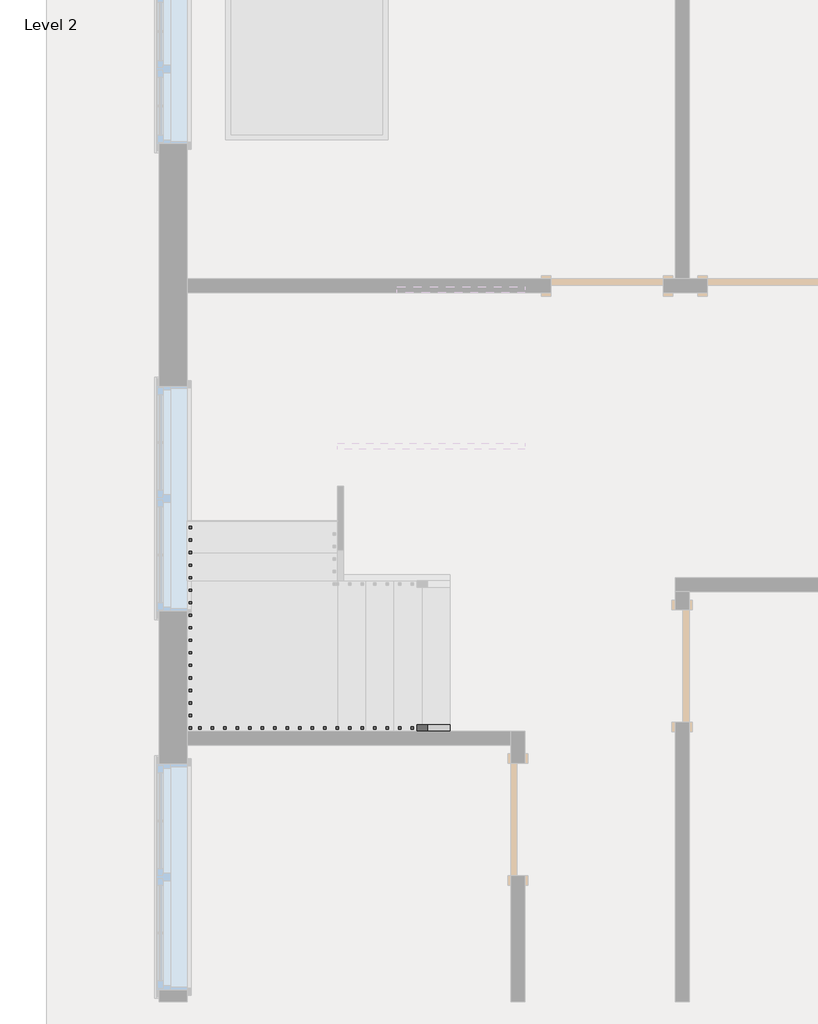
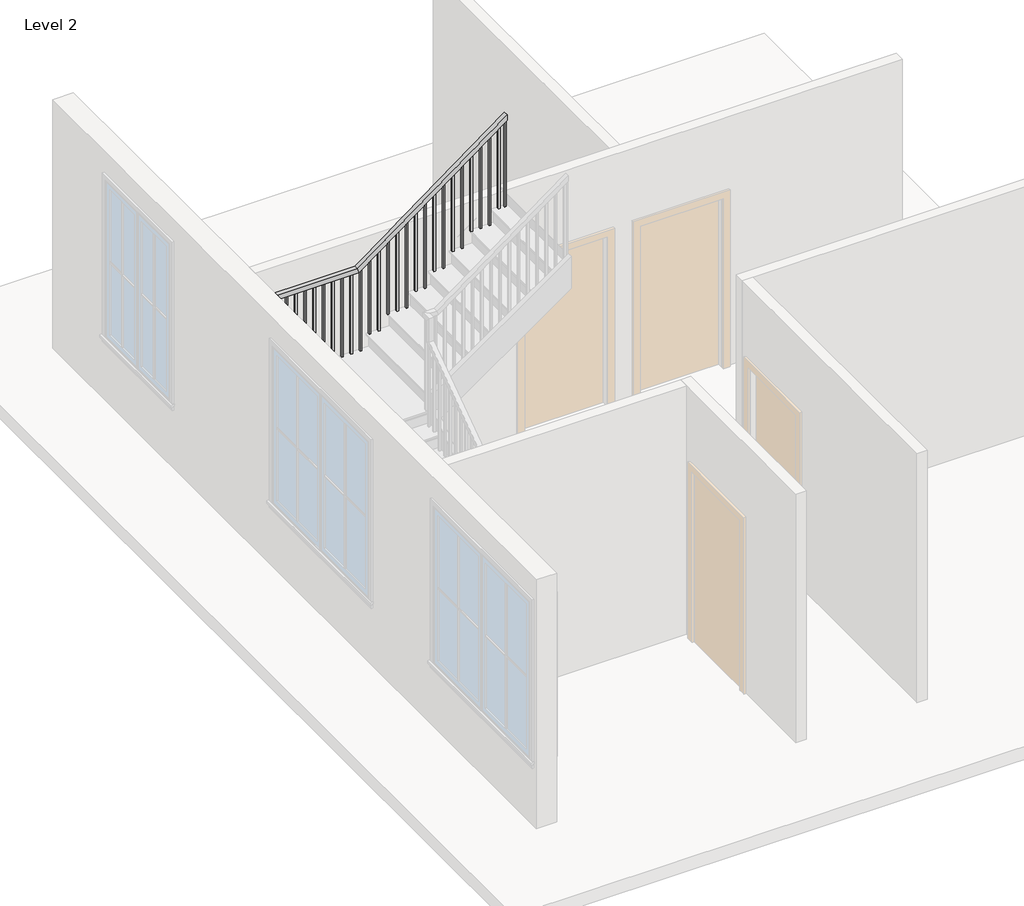
# One storey, part 2 of 3: 1 railing.
"""IFC4 building model written with IfcOpenShell, lengths in millimetres."""

from ifc_helpers import new_model, si_unit, frame, origin, place, context, project, spatial, polyline, outline, extrude, faceted_brep, element, save

model = new_model("IFC4")

# Units and contexts
model_context = context("Model", 3, world=origin())
ifc_project = project(units=[si_unit("LENGTHUNIT", "METRE", prefix="MILLI")], contexts=[model_context])

# Site, building, storey
site = spatial("IfcSite", under=ifc_project)
building = spatial("IfcBuilding", under=site)
storey = spatial("IfcBuildingStorey", under=building, Name="Level 2", Elevation=3048.0)

# Railing
placement = place(None, origin())
element("IfcRailing", 1, ObjectType="Handrail - Rectangular", at=placement, inside=storey, context=model_context, shape_type="SolidModel", body=[
    faceted_brep([(-2683.1105391, -2741.0373761, 4122.8210526), (-2683.1105391, -2741.0373761, 4060.7605986), (-2683.1105391, -2690.2373761, 4060.7605986), (-2683.1105391, -2690.2373761, 4122.8210526), (-3698.24463, -2741.0373761, 4835.1958533), (-3714.290777, -2741.0373761, 4784.3958533), (-3714.290777, -2690.2373761, 4784.3958533), (-3698.24463, -2690.2373761, 4835.1958533), (-4816.7105391, -2741.0373761, 4835.1958533), (-4816.7105391, -2741.0373761, 4784.3958533), (-4765.9105391, -2690.2373761, 4784.3958533), (-4765.9105391, -2690.2373761, 4835.1958533), (-4816.7105391, -1646.8618205, 4835.1958533), (-4816.7105391, -1630.5188912, 4784.3958533), (-4765.9105391, -1630.5188912, 4784.3958533), (-4765.9105391, -1646.8618205, 4835.1958533), (-4816.7105391, -308.3947094, 5795.8181818), (-4816.7105391, -292.0517801, 5745.0181818), (-4765.9105391, -292.0517801, 5745.0181818), (-4765.9105391, -308.3947094, 5795.8181818), (-4816.7105391, 814.9626239, 5795.8181818), (-4816.7105391, 814.9626239, 5745.0181818), (-4765.9105391, 764.1626239, 5745.0181818), (-4765.9105391, 764.1626239, 5795.8181818), (-3721.871578, 814.9626239, 5795.8181818), (-3705.1770744, 814.9626239, 5745.0181818), (-3705.1770744, 764.1626239, 5745.0181818), (-3721.871578, 764.1626239, 5795.8181818), (-2073.5105391, 814.9626239, 7010.4), (-2073.5105391, 764.1626239, 7010.4), (-2073.5105391, 764.1626239, 6947.2987868), (-2073.5105391, 814.9626239, 6947.2987868)], [[[0, 1, 2, 3]], [[1, 0, 4, 5]], [[2, 1, 5, 6]], [[3, 2, 6, 7]], [[0, 3, 7, 4]], [[5, 4, 8, 9]], [[6, 5, 9, 10]], [[7, 6, 10, 11]], [[4, 7, 11, 8]], [[9, 8, 12, 13]], [[10, 9, 13, 14]], [[11, 10, 14, 15]], [[8, 11, 15, 12]], [[13, 12, 16, 17]], [[14, 13, 17, 18]], [[15, 14, 18, 19]], [[12, 15, 19, 16]], [[17, 16, 20, 21]], [[18, 17, 21, 22]], [[19, 18, 22, 23]], [[16, 19, 23, 20]], [[21, 20, 24, 25]], [[22, 21, 25, 26]], [[23, 22, 26, 27]], [[20, 23, 27, 24]], [[28, 29, 30, 31]], [[25, 24, 28, 31]], [[26, 25, 31, 30]], [[27, 26, 30, 29]], [[24, 27, 29, 28]]]),
    extrude(outline(polyline([(6884.1329974, -2159.2355391), (5935.5789474, -2159.2355391), (5935.5789474, -2140.1855391), (6898.1698395, -2140.1855391), (6884.1329974, -2159.2355391)])), frame((0.0, 780.0376239, 0.0), z_axis=(0.0, 1.0, 0.0), x_axis=(0.0, 0.0, 1.0)), (0.0, 0.0, 1.0), 19.05),
    extrude(outline(polyline([(6809.2698395, -2260.8355391), (5775.1578947, -2260.8355391), (5775.1578947, -2241.7855391), (6823.3066816, -2241.7855391), (6809.2698395, -2260.8355391)])), frame((0.0, 780.0376239, 0.0), z_axis=(0.0, 1.0, 0.0), x_axis=(0.0, 0.0, 1.0)), (0.0, 0.0, 1.0), 19.05),
    extrude(outline(polyline([(6734.4066816, -2362.4355391), (5775.1578947, -2362.4355391), (5775.1578947, -2343.3855391), (6748.4435237, -2343.3855391), (6734.4066816, -2362.4355391)])), frame((0.0, 780.0376239, 0.0), z_axis=(0.0, 1.0, 0.0), x_axis=(0.0, 0.0, 1.0)), (0.0, 0.0, 1.0), 19.05),
    extrude(outline(polyline([(6659.5435237, -2464.0355391), (5775.1578947, -2464.0355391), (5775.1578947, -2444.9855391), (6673.5803658, -2444.9855391), (6659.5435237, -2464.0355391)])), frame((0.0, 780.0376239, 0.0), z_axis=(0.0, 1.0, 0.0), x_axis=(0.0, 0.0, 1.0)), (0.0, 0.0, 1.0), 19.05),
    extrude(outline(polyline([(6584.6803658, -2565.6355391), (5614.7368421, -2565.6355391), (5614.7368421, -2546.5855391), (6598.7172079, -2546.5855391), (6584.6803658, -2565.6355391)])), frame((0.0, 780.0376239, 0.0), z_axis=(0.0, 1.0, 0.0), x_axis=(0.0, 0.0, 1.0)), (0.0, 0.0, 1.0), 19.05),
    extrude(outline(polyline([(6509.8172079, -2667.2355391), (5614.7368421, -2667.2355391), (5614.7368421, -2648.1855391), (6523.85405, -2648.1855391), (6509.8172079, -2667.2355391)])), frame((0.0, 780.0376239, 0.0), z_axis=(0.0, 1.0, 0.0), x_axis=(0.0, 0.0, 1.0)), (0.0, 0.0, 1.0), 19.05),
    extrude(outline(polyline([(6434.95405, -2768.8355391), (5454.3157895, -2768.8355391), (5454.3157895, -2749.7855391), (6448.9908921, -2749.7855391), (6434.95405, -2768.8355391)])), frame((0.0, 780.0376239, 0.0), z_axis=(0.0, 1.0, 0.0), x_axis=(0.0, 0.0, 1.0)), (0.0, 0.0, 1.0), 19.05),
    extrude(outline(polyline([(6360.0908921, -2870.4355391), (5454.3157895, -2870.4355391), (5454.3157895, -2851.3855391), (6374.1277342, -2851.3855391), (6360.0908921, -2870.4355391)])), frame((0.0, 780.0376239, 0.0), z_axis=(0.0, 1.0, 0.0), x_axis=(0.0, 0.0, 1.0)), (0.0, 0.0, 1.0), 19.05),
    extrude(outline(polyline([(6285.2277342, -2972.0355391), (5293.8947368, -2972.0355391), (5293.8947368, -2952.9855391), (6299.2645763, -2952.9855391), (6285.2277342, -2972.0355391)])), frame((0.0, 780.0376239, 0.0), z_axis=(0.0, 1.0, 0.0), x_axis=(0.0, 0.0, 1.0)), (0.0, 0.0, 1.0), 19.05),
    extrude(outline(polyline([(6210.3645763, -3073.6355391), (5293.8947368, -3073.6355391), (5293.8947368, -3054.5855391), (6224.4014184, -3054.5855391), (6210.3645763, -3073.6355391)])), frame((0.0, 780.0376239, 0.0), z_axis=(0.0, 1.0, 0.0), x_axis=(0.0, 0.0, 1.0)), (0.0, 0.0, 1.0), 19.05),
    extrude(outline(polyline([(6135.5014184, -3175.2355391), (5133.4736842, -3175.2355391), (5133.4736842, -3156.1855391), (6149.5382605, -3156.1855391), (6135.5014184, -3175.2355391)])), frame((0.0, 780.0376239, 0.0), z_axis=(0.0, 1.0, 0.0), x_axis=(0.0, 0.0, 1.0)), (0.0, 0.0, 1.0), 19.05),
    extrude(outline(polyline([(6060.6382605, -3276.8355391), (5133.4736842, -3276.8355391), (5133.4736842, -3257.7855391), (6074.6751026, -3257.7855391), (6060.6382605, -3276.8355391)])), frame((0.0, 780.0376239, 0.0), z_axis=(0.0, 1.0, 0.0), x_axis=(0.0, 0.0, 1.0)), (0.0, 0.0, 1.0), 19.05),
    extrude(outline(polyline([(5985.7751026, -3378.4355391), (5133.4736842, -3378.4355391), (5133.4736842, -3359.3855391), (5999.8119447, -3359.3855391), (5985.7751026, -3378.4355391)])), frame((0.0, 780.0376239, 0.0), z_axis=(0.0, 1.0, 0.0), x_axis=(0.0, 0.0, 1.0)), (0.0, 0.0, 1.0), 19.05),
    extrude(outline(polyline([(5910.9119447, -3480.0355391), (4973.0526316, -3480.0355391), (4973.0526316, -3460.9855391), (5924.9487868, -3460.9855391), (5910.9119447, -3480.0355391)])), frame((0.0, 780.0376239, 0.0), z_axis=(0.0, 1.0, 0.0), x_axis=(0.0, 0.0, 1.0)), (0.0, 0.0, 1.0), 19.05),
    extrude(outline(polyline([(5836.0487868, -3581.6355391), (4973.0526316, -3581.6355391), (4973.0526316, -3562.5855391), (5850.0856289, -3562.5855391), (5836.0487868, -3581.6355391)])), frame((0.0, 780.0376239, 0.0), z_axis=(0.0, 1.0, 0.0), x_axis=(0.0, 0.0, 1.0)), (0.0, 0.0, 1.0), 19.05),
    extrude(outline(polyline([(5761.1856289, -3683.2355391), (4812.6315789, -3683.2355391), (4812.6315789, -3664.1855391), (5775.222471, -3664.1855391), (5761.1856289, -3683.2355391)])), frame((0.0, 780.0376239, 0.0), z_axis=(0.0, 1.0, 0.0), x_axis=(0.0, 0.0, 1.0)), (0.0, 0.0, 1.0), 19.05),
    extrude(outline(polyline([(-3784.8355391, 799.0876239), (-3765.7855391, 799.0876239), (-3765.7855391, 780.0376239), (-3784.8355391, 780.0376239), (-3784.8355391, 799.0876239)])), frame((0.0, 0.0, 4812.6315789), z_axis=(0.0, 0.0, 1.0), x_axis=(1.0, 0.0, 0.0)), (0.0, 0.0, 1.0), 932.3866029),
    extrude(outline(polyline([(-3886.4355391, 799.0876239), (-3867.3855391, 799.0876239), (-3867.3855391, 780.0376239), (-3886.4355391, 780.0376239), (-3886.4355391, 799.0876239)])), frame((0.0, 0.0, 4812.6315789), z_axis=(0.0, 0.0, 1.0), x_axis=(1.0, 0.0, 0.0)), (0.0, 0.0, 1.0), 932.3866029),
    extrude(outline(polyline([(-3988.0355391, 799.0876239), (-3968.9855391, 799.0876239), (-3968.9855391, 780.0376239), (-3988.0355391, 780.0376239), (-3988.0355391, 799.0876239)])), frame((0.0, 0.0, 4812.6315789), z_axis=(0.0, 0.0, 1.0), x_axis=(1.0, 0.0, 0.0)), (0.0, 0.0, 1.0), 932.3866029),
    extrude(outline(polyline([(-4089.6355391, 799.0876239), (-4070.5855391, 799.0876239), (-4070.5855391, 780.0376239), (-4089.6355391, 780.0376239), (-4089.6355391, 799.0876239)])), frame((0.0, 0.0, 4812.6315789), z_axis=(0.0, 0.0, 1.0), x_axis=(1.0, 0.0, 0.0)), (0.0, 0.0, 1.0), 932.3866029),
    extrude(outline(polyline([(-4191.2355391, 799.0876239), (-4172.1855391, 799.0876239), (-4172.1855391, 780.0376239), (-4191.2355391, 780.0376239), (-4191.2355391, 799.0876239)])), frame((0.0, 0.0, 4812.6315789), z_axis=(0.0, 0.0, 1.0), x_axis=(1.0, 0.0, 0.0)), (0.0, 0.0, 1.0), 932.3866029),
    extrude(outline(polyline([(-4292.8355391, 799.0876239), (-4273.7855391, 799.0876239), (-4273.7855391, 780.0376239), (-4292.8355391, 780.0376239), (-4292.8355391, 799.0876239)])), frame((0.0, 0.0, 4812.6315789), z_axis=(0.0, 0.0, 1.0), x_axis=(1.0, 0.0, 0.0)), (0.0, 0.0, 1.0), 932.3866029),
    extrude(outline(polyline([(-4394.4355391, 799.0876239), (-4375.3855391, 799.0876239), (-4375.3855391, 780.0376239), (-4394.4355391, 780.0376239), (-4394.4355391, 799.0876239)])), frame((0.0, 0.0, 4812.6315789), z_axis=(0.0, 0.0, 1.0), x_axis=(1.0, 0.0, 0.0)), (0.0, 0.0, 1.0), 932.3866029),
    extrude(outline(polyline([(-4496.0355391, 799.0876239), (-4476.9855391, 799.0876239), (-4476.9855391, 780.0376239), (-4496.0355391, 780.0376239), (-4496.0355391, 799.0876239)])), frame((0.0, 0.0, 4812.6315789), z_axis=(0.0, 0.0, 1.0), x_axis=(1.0, 0.0, 0.0)), (0.0, 0.0, 1.0), 932.3866029),
    extrude(outline(polyline([(-4597.6355391, 799.0876239), (-4578.5855391, 799.0876239), (-4578.5855391, 780.0376239), (-4597.6355391, 780.0376239), (-4597.6355391, 799.0876239)])), frame((0.0, 0.0, 4812.6315789), z_axis=(0.0, 0.0, 1.0), x_axis=(1.0, 0.0, 0.0)), (0.0, 0.0, 1.0), 932.3866029),
    extrude(outline(polyline([(-4699.2355391, 799.0876239), (-4680.1855391, 799.0876239), (-4680.1855391, 780.0376239), (-4699.2355391, 780.0376239), (-4699.2355391, 799.0876239)])), frame((0.0, 0.0, 4812.6315789), z_axis=(0.0, 0.0, 1.0), x_axis=(1.0, 0.0, 0.0)), (0.0, 0.0, 1.0), 932.3866029),
    extrude(outline(polyline([(-4800.8355391, 729.2376239), (-4800.8355391, 748.2876239), (-4781.7855391, 748.2876239), (-4781.7855391, 729.2376239), (-4800.8355391, 729.2376239)])), frame((0.0, 0.0, 4812.6315789), z_axis=(0.0, 0.0, 1.0), x_axis=(1.0, 0.0, 0.0)), (0.0, 0.0, 1.0), 932.3866029),
    extrude(outline(polyline([(-4800.8355391, 627.6376239), (-4800.8355391, 646.6876239), (-4781.7855391, 646.6876239), (-4781.7855391, 627.6376239), (-4800.8355391, 627.6376239)])), frame((0.0, 0.0, 4812.6315789), z_axis=(0.0, 0.0, 1.0), x_axis=(1.0, 0.0, 0.0)), (0.0, 0.0, 1.0), 932.3866029),
    extrude(outline(polyline([(-4800.8355391, 526.0376239), (-4800.8355391, 545.0876239), (-4781.7855391, 545.0876239), (-4781.7855391, 526.0376239), (-4800.8355391, 526.0376239)])), frame((0.0, 0.0, 4812.6315789), z_axis=(0.0, 0.0, 1.0), x_axis=(1.0, 0.0, 0.0)), (0.0, 0.0, 1.0), 932.3866029),
    extrude(outline(polyline([(-4800.8355391, 424.4376239), (-4800.8355391, 443.4876239), (-4781.7855391, 443.4876239), (-4781.7855391, 424.4376239), (-4800.8355391, 424.4376239)])), frame((0.0, 0.0, 4812.6315789), z_axis=(0.0, 0.0, 1.0), x_axis=(1.0, 0.0, 0.0)), (0.0, 0.0, 1.0), 932.3866029),
    extrude(outline(polyline([(-4800.8355391, 322.8376239), (-4800.8355391, 341.8876239), (-4781.7855391, 341.8876239), (-4781.7855391, 322.8376239), (-4800.8355391, 322.8376239)])), frame((0.0, 0.0, 4812.6315789), z_axis=(0.0, 0.0, 1.0), x_axis=(1.0, 0.0, 0.0)), (0.0, 0.0, 1.0), 932.3866029),
    extrude(outline(polyline([(-4800.8355391, 221.2376239), (-4800.8355391, 240.2876239), (-4781.7855391, 240.2876239), (-4781.7855391, 221.2376239), (-4800.8355391, 221.2376239)])), frame((0.0, 0.0, 4812.6315789), z_axis=(0.0, 0.0, 1.0), x_axis=(1.0, 0.0, 0.0)), (0.0, 0.0, 1.0), 932.3866029),
    extrude(outline(polyline([(-4800.8355391, 119.6376239), (-4800.8355391, 138.6876239), (-4781.7855391, 138.6876239), (-4781.7855391, 119.6376239), (-4800.8355391, 119.6376239)])), frame((0.0, 0.0, 4812.6315789), z_axis=(0.0, 0.0, 1.0), x_axis=(1.0, 0.0, 0.0)), (0.0, 0.0, 1.0), 932.3866029),
    extrude(outline(polyline([(-4800.8355391, 18.0376239), (-4800.8355391, 37.0876239), (-4781.7855391, 37.0876239), (-4781.7855391, 18.0376239), (-4800.8355391, 18.0376239)])), frame((0.0, 0.0, 4812.6315789), z_axis=(0.0, 0.0, 1.0), x_axis=(1.0, 0.0, 0.0)), (0.0, 0.0, 1.0), 932.3866029),
    extrude(outline(polyline([(-4800.8355391, -83.5623761), (-4800.8355391, -64.5123761), (-4781.7855391, -64.5123761), (-4781.7855391, -83.5623761), (-4800.8355391, -83.5623761)])), frame((0.0, 0.0, 4812.6315789), z_axis=(0.0, 0.0, 1.0), x_axis=(1.0, 0.0, 0.0)), (0.0, 0.0, 1.0), 932.3866029),
    extrude(outline(polyline([(-4800.8355391, -185.1623761), (-4800.8355391, -166.1123761), (-4781.7855391, -166.1123761), (-4781.7855391, -185.1623761), (-4800.8355391, -185.1623761)])), frame((0.0, 0.0, 4812.6315789), z_axis=(0.0, 0.0, 1.0), x_axis=(1.0, 0.0, 0.0)), (0.0, 0.0, 1.0), 932.3866029),
    extrude(outline(polyline([(-4800.8355391, -286.7623761), (-4800.8355391, -267.7123761), (-4781.7855391, -267.7123761), (-4781.7855391, -286.7623761), (-4800.8355391, -286.7623761)])), frame((0.0, 0.0, 4812.6315789), z_axis=(0.0, 0.0, 1.0), x_axis=(1.0, 0.0, 0.0)), (0.0, 0.0, 1.0), 932.3866029),
    extrude(outline(polyline([(-369.3123761, 5689.5679933), (-369.3123761, 4812.6315789), (-388.3623761, 4812.6315789), (-388.3623761, 5675.8957445), (-369.3123761, 5689.5679933)])), frame((-4800.8355391, 0.0, 0.0), z_axis=(1.0, 0.0, 0.0), x_axis=(0.0, 1.0, 0.0)), (0.0, 0.0, 1.0), 19.05),
    extrude(outline(polyline([(-470.9123761, 5616.649333), (-470.9123761, 4652.2105263), (-489.9623761, 4652.2105263), (-489.9623761, 5602.9770842), (-470.9123761, 5616.649333)])), frame((-4800.8355391, 0.0, 0.0), z_axis=(1.0, 0.0, 0.0), x_axis=(0.0, 1.0, 0.0)), (0.0, 0.0, 1.0), 19.05),
    extrude(outline(polyline([(-572.5123761, 5543.7306727), (-572.5123761, 4652.2105263), (-591.5623761, 4652.2105263), (-591.5623761, 5530.0584239), (-572.5123761, 5543.7306727)])), frame((-4800.8355391, 0.0, 0.0), z_axis=(1.0, 0.0, 0.0), x_axis=(0.0, 1.0, 0.0)), (0.0, 0.0, 1.0), 19.05),
    extrude(outline(polyline([(-674.1123761, 5470.8120124), (-674.1123761, 4491.7894737), (-693.1623761, 4491.7894737), (-693.1623761, 5457.1397636), (-674.1123761, 5470.8120124)])), frame((-4800.8355391, 0.0, 0.0), z_axis=(1.0, 0.0, 0.0), x_axis=(0.0, 1.0, 0.0)), (0.0, 0.0, 1.0), 19.05),
    extrude(outline(polyline([(-775.7123761, 5397.8933521), (-775.7123761, 4491.7894737), (-794.7623761, 4491.7894737), (-794.7623761, 5384.2211033), (-775.7123761, 5397.8933521)])), frame((-4800.8355391, 0.0, 0.0), z_axis=(1.0, 0.0, 0.0), x_axis=(0.0, 1.0, 0.0)), (0.0, 0.0, 1.0), 19.05),
    extrude(outline(polyline([(-877.3123761, 5324.9746919), (-877.3123761, 4331.3684211), (-896.3623761, 4331.3684211), (-896.3623761, 5311.302443), (-877.3123761, 5324.9746919)])), frame((-4800.8355391, 0.0, 0.0), z_axis=(1.0, 0.0, 0.0), x_axis=(0.0, 1.0, 0.0)), (0.0, 0.0, 1.0), 19.05),
    extrude(outline(polyline([(-978.9123761, 5252.0560316), (-978.9123761, 4331.3684211), (-997.9623761, 4331.3684211), (-997.9623761, 5238.3837828), (-978.9123761, 5252.0560316)])), frame((-4800.8355391, 0.0, 0.0), z_axis=(1.0, 0.0, 0.0), x_axis=(0.0, 1.0, 0.0)), (0.0, 0.0, 1.0), 19.05),
    extrude(outline(polyline([(-1080.5123761, 5179.1373713), (-1080.5123761, 4170.9473684), (-1099.5623761, 4170.9473684), (-1099.5623761, 5165.4651225), (-1080.5123761, 5179.1373713)])), frame((-4800.8355391, 0.0, 0.0), z_axis=(1.0, 0.0, 0.0), x_axis=(0.0, 1.0, 0.0)), (0.0, 0.0, 1.0), 19.05),
    extrude(outline(polyline([(-1182.1123761, 5106.218711), (-1182.1123761, 4170.9473684), (-1201.1623761, 4170.9473684), (-1201.1623761, 5092.5464622), (-1182.1123761, 5106.218711)])), frame((-4800.8355391, 0.0, 0.0), z_axis=(1.0, 0.0, 0.0), x_axis=(0.0, 1.0, 0.0)), (0.0, 0.0, 1.0), 19.05),
    extrude(outline(polyline([(-1283.7123761, 5033.3000507), (-1283.7123761, 4170.9473684), (-1302.7623761, 4170.9473684), (-1302.7623761, 5019.6278019), (-1283.7123761, 5033.3000507)])), frame((-4800.8355391, 0.0, 0.0), z_axis=(1.0, 0.0, 0.0), x_axis=(0.0, 1.0, 0.0)), (0.0, 0.0, 1.0), 19.05),
    extrude(outline(polyline([(-1385.3123761, 4960.3813904), (-1385.3123761, 4010.5263158), (-1404.3623761, 4010.5263158), (-1404.3623761, 4946.7091416), (-1385.3123761, 4960.3813904)])), frame((-4800.8355391, 0.0, 0.0), z_axis=(1.0, 0.0, 0.0), x_axis=(0.0, 1.0, 0.0)), (0.0, 0.0, 1.0), 19.05),
    extrude(outline(polyline([(-1486.9123761, 4887.4627301), (-1486.9123761, 4010.5263158), (-1505.9623761, 4010.5263158), (-1505.9623761, 4873.7904813), (-1486.9123761, 4887.4627301)])), frame((-4800.8355391, 0.0, 0.0), z_axis=(1.0, 0.0, 0.0), x_axis=(0.0, 1.0, 0.0)), (0.0, 0.0, 1.0), 19.05),
    extrude(outline(polyline([(-1588.5123761, 4814.5440698), (-1588.5123761, 3850.1052632), (-1607.5623761, 3850.1052632), (-1607.5623761, 4800.871821), (-1588.5123761, 4814.5440698)])), frame((-4800.8355391, 0.0, 0.0), z_axis=(1.0, 0.0, 0.0), x_axis=(0.0, 1.0, 0.0)), (0.0, 0.0, 1.0), 19.05),
    extrude(outline(polyline([(-4800.8355391, -1709.1623761), (-4800.8355391, -1690.1123761), (-4781.7855391, -1690.1123761), (-4781.7855391, -1709.1623761), (-4800.8355391, -1709.1623761)])), frame((0.0, 0.0, 3850.1052632), z_axis=(0.0, 0.0, 1.0), x_axis=(1.0, 0.0, 0.0)), (0.0, 0.0, 1.0), 934.2905901),
    extrude(outline(polyline([(-4800.8355391, -1810.7623761), (-4800.8355391, -1791.7123761), (-4781.7855391, -1791.7123761), (-4781.7855391, -1810.7623761), (-4800.8355391, -1810.7623761)])), frame((0.0, 0.0, 3850.1052632), z_axis=(0.0, 0.0, 1.0), x_axis=(1.0, 0.0, 0.0)), (0.0, 0.0, 1.0), 934.2905901),
    extrude(outline(polyline([(-4800.8355391, -1912.3623761), (-4800.8355391, -1893.3123761), (-4781.7855391, -1893.3123761), (-4781.7855391, -1912.3623761), (-4800.8355391, -1912.3623761)])), frame((0.0, 0.0, 3850.1052632), z_axis=(0.0, 0.0, 1.0), x_axis=(1.0, 0.0, 0.0)), (0.0, 0.0, 1.0), 934.2905901),
    extrude(outline(polyline([(-4800.8355391, -2013.9623761), (-4800.8355391, -1994.9123761), (-4781.7855391, -1994.9123761), (-4781.7855391, -2013.9623761), (-4800.8355391, -2013.9623761)])), frame((0.0, 0.0, 3850.1052632), z_axis=(0.0, 0.0, 1.0), x_axis=(1.0, 0.0, 0.0)), (0.0, 0.0, 1.0), 934.2905901),
    extrude(outline(polyline([(-4800.8355391, -2115.5623761), (-4800.8355391, -2096.5123761), (-4781.7855391, -2096.5123761), (-4781.7855391, -2115.5623761), (-4800.8355391, -2115.5623761)])), frame((0.0, 0.0, 3850.1052632), z_axis=(0.0, 0.0, 1.0), x_axis=(1.0, 0.0, 0.0)), (0.0, 0.0, 1.0), 934.2905901),
    extrude(outline(polyline([(-4800.8355391, -2217.1623761), (-4800.8355391, -2198.1123761), (-4781.7855391, -2198.1123761), (-4781.7855391, -2217.1623761), (-4800.8355391, -2217.1623761)])), frame((0.0, 0.0, 3850.1052632), z_axis=(0.0, 0.0, 1.0), x_axis=(1.0, 0.0, 0.0)), (0.0, 0.0, 1.0), 934.2905901),
    extrude(outline(polyline([(-4800.8355391, -2318.7623761), (-4800.8355391, -2299.7123761), (-4781.7855391, -2299.7123761), (-4781.7855391, -2318.7623761), (-4800.8355391, -2318.7623761)])), frame((0.0, 0.0, 3850.1052632), z_axis=(0.0, 0.0, 1.0), x_axis=(1.0, 0.0, 0.0)), (0.0, 0.0, 1.0), 934.2905901),
    extrude(outline(polyline([(-4800.8355391, -2420.3623761), (-4800.8355391, -2401.3123761), (-4781.7855391, -2401.3123761), (-4781.7855391, -2420.3623761), (-4800.8355391, -2420.3623761)])), frame((0.0, 0.0, 3850.1052632), z_axis=(0.0, 0.0, 1.0), x_axis=(1.0, 0.0, 0.0)), (0.0, 0.0, 1.0), 934.2905901),
    extrude(outline(polyline([(-4800.8355391, -2521.9623761), (-4800.8355391, -2502.9123761), (-4781.7855391, -2502.9123761), (-4781.7855391, -2521.9623761), (-4800.8355391, -2521.9623761)])), frame((0.0, 0.0, 3850.1052632), z_axis=(0.0, 0.0, 1.0), x_axis=(1.0, 0.0, 0.0)), (0.0, 0.0, 1.0), 934.2905901),
    extrude(outline(polyline([(-4800.8355391, -2623.5623761), (-4800.8355391, -2604.5123761), (-4781.7855391, -2604.5123761), (-4781.7855391, -2623.5623761), (-4800.8355391, -2623.5623761)])), frame((0.0, 0.0, 3850.1052632), z_axis=(0.0, 0.0, 1.0), x_axis=(1.0, 0.0, 0.0)), (0.0, 0.0, 1.0), 934.2905901),
    extrude(outline(polyline([(-4705.5855391, -2725.1623761), (-4724.6355391, -2725.1623761), (-4724.6355391, -2706.1123761), (-4705.5855391, -2706.1123761), (-4705.5855391, -2725.1623761)])), frame((0.0, 0.0, 3850.1052632), z_axis=(0.0, 0.0, 1.0), x_axis=(1.0, 0.0, 0.0)), (0.0, 0.0, 1.0), 934.2905901),
    extrude(outline(polyline([(-4603.9855391, -2725.1623761), (-4623.0355391, -2725.1623761), (-4623.0355391, -2706.1123761), (-4603.9855391, -2706.1123761), (-4603.9855391, -2725.1623761)])), frame((0.0, 0.0, 3850.1052632), z_axis=(0.0, 0.0, 1.0), x_axis=(1.0, 0.0, 0.0)), (0.0, 0.0, 1.0), 934.2905901),
    extrude(outline(polyline([(-4502.3855391, -2725.1623761), (-4521.4355391, -2725.1623761), (-4521.4355391, -2706.1123761), (-4502.3855391, -2706.1123761), (-4502.3855391, -2725.1623761)])), frame((0.0, 0.0, 3850.1052632), z_axis=(0.0, 0.0, 1.0), x_axis=(1.0, 0.0, 0.0)), (0.0, 0.0, 1.0), 934.2905901),
    extrude(outline(polyline([(-4400.7855391, -2725.1623761), (-4419.8355391, -2725.1623761), (-4419.8355391, -2706.1123761), (-4400.7855391, -2706.1123761), (-4400.7855391, -2725.1623761)])), frame((0.0, 0.0, 3850.1052632), z_axis=(0.0, 0.0, 1.0), x_axis=(1.0, 0.0, 0.0)), (0.0, 0.0, 1.0), 934.2905901),
    extrude(outline(polyline([(-4299.1855391, -2725.1623761), (-4318.2355391, -2725.1623761), (-4318.2355391, -2706.1123761), (-4299.1855391, -2706.1123761), (-4299.1855391, -2725.1623761)])), frame((0.0, 0.0, 3850.1052632), z_axis=(0.0, 0.0, 1.0), x_axis=(1.0, 0.0, 0.0)), (0.0, 0.0, 1.0), 934.2905901),
    extrude(outline(polyline([(-4197.5855391, -2725.1623761), (-4216.6355391, -2725.1623761), (-4216.6355391, -2706.1123761), (-4197.5855391, -2706.1123761), (-4197.5855391, -2725.1623761)])), frame((0.0, 0.0, 3850.1052632), z_axis=(0.0, 0.0, 1.0), x_axis=(1.0, 0.0, 0.0)), (0.0, 0.0, 1.0), 934.2905901),
    extrude(outline(polyline([(-4095.9855391, -2725.1623761), (-4115.0355391, -2725.1623761), (-4115.0355391, -2706.1123761), (-4095.9855391, -2706.1123761), (-4095.9855391, -2725.1623761)])), frame((0.0, 0.0, 3850.1052632), z_axis=(0.0, 0.0, 1.0), x_axis=(1.0, 0.0, 0.0)), (0.0, 0.0, 1.0), 934.2905901),
    extrude(outline(polyline([(-3994.3855391, -2725.1623761), (-4013.4355391, -2725.1623761), (-4013.4355391, -2706.1123761), (-3994.3855391, -2706.1123761), (-3994.3855391, -2725.1623761)])), frame((0.0, 0.0, 3850.1052632), z_axis=(0.0, 0.0, 1.0), x_axis=(1.0, 0.0, 0.0)), (0.0, 0.0, 1.0), 934.2905901),
    extrude(outline(polyline([(-3892.7855391, -2725.1623761), (-3911.8355391, -2725.1623761), (-3911.8355391, -2706.1123761), (-3892.7855391, -2706.1123761), (-3892.7855391, -2725.1623761)])), frame((0.0, 0.0, 3850.1052632), z_axis=(0.0, 0.0, 1.0), x_axis=(1.0, 0.0, 0.0)), (0.0, 0.0, 1.0), 934.2905901),
    extrude(outline(polyline([(-3791.1855391, -2725.1623761), (-3810.2355391, -2725.1623761), (-3810.2355391, -2706.1123761), (-3791.1855391, -2706.1123761), (-3791.1855391, -2725.1623761)])), frame((0.0, 0.0, 3850.1052632), z_axis=(0.0, 0.0, 1.0), x_axis=(1.0, 0.0, 0.0)), (0.0, 0.0, 1.0), 934.2905901),
    extrude(outline(polyline([(-3689.5855391, -2725.1623761), (-3708.6355391, -2725.1623761), (-3708.6355391, -2706.1123761), (-3689.5855391, -2706.1123761), (-3689.5855391, -2725.1623761)])), frame((0.0, 0.0, 3850.1052632), z_axis=(0.0, 0.0, 1.0), x_axis=(1.0, 0.0, 0.0)), (0.0, 0.0, 1.0), 934.2905901),
    extrude(outline(polyline([(4709.1290196, -3607.0355391), (3850.1052632, -3607.0355391), (3850.1052632, -3587.9855391), (4695.7605986, -3587.9855391), (4709.1290196, -3607.0355391)])), frame((0.0, -2725.1623761, 0.0), z_axis=(0.0, 1.0, 0.0), x_axis=(0.0, 0.0, 1.0)), (0.0, 0.0, 1.0), 19.05),
    extrude(outline(polyline([(4637.830774, -3505.4355391), (3689.6842105, -3505.4355391), (3689.6842105, -3486.3855391), (4624.462353, -3486.3855391), (4637.830774, -3505.4355391)])), frame((0.0, -2725.1623761, 0.0), z_axis=(0.0, 1.0, 0.0), x_axis=(0.0, 0.0, 1.0)), (0.0, 0.0, 1.0), 19.05),
    extrude(outline(polyline([(4566.5325284, -3403.8355391), (3689.6842105, -3403.8355391), (3689.6842105, -3384.7855391), (4553.1641074, -3384.7855391), (4566.5325284, -3403.8355391)])), frame((0.0, -2725.1623761, 0.0), z_axis=(0.0, 1.0, 0.0), x_axis=(0.0, 0.0, 1.0)), (0.0, 0.0, 1.0), 19.05),
    extrude(outline(polyline([(4495.2342828, -3302.2355391), (3529.2631579, -3302.2355391), (3529.2631579, -3283.1855391), (4481.8658617, -3283.1855391), (4495.2342828, -3302.2355391)])), frame((0.0, -2725.1623761, 0.0), z_axis=(0.0, 1.0, 0.0), x_axis=(0.0, 0.0, 1.0)), (0.0, 0.0, 1.0), 19.05),
    extrude(outline(polyline([(4423.9360372, -3200.6355391), (3529.2631579, -3200.6355391), (3529.2631579, -3181.5855391), (4410.5676161, -3181.5855391), (4423.9360372, -3200.6355391)])), frame((0.0, -2725.1623761, 0.0), z_axis=(0.0, 1.0, 0.0), x_axis=(0.0, 0.0, 1.0)), (0.0, 0.0, 1.0), 19.05),
    extrude(outline(polyline([(4352.6377916, -3099.0355391), (3368.8421053, -3099.0355391), (3368.8421053, -3079.9855391), (4339.2693705, -3079.9855391), (4352.6377916, -3099.0355391)])), frame((0.0, -2725.1623761, 0.0), z_axis=(0.0, 1.0, 0.0), x_axis=(0.0, 0.0, 1.0)), (0.0, 0.0, 1.0), 19.05),
    extrude(outline(polyline([(4281.3395459, -2997.4355391), (3368.8421053, -2997.4355391), (3368.8421053, -2978.3855391), (4267.9711249, -2978.3855391), (4281.3395459, -2997.4355391)])), frame((0.0, -2725.1623761, 0.0), z_axis=(0.0, 1.0, 0.0), x_axis=(0.0, 0.0, 1.0)), (0.0, 0.0, 1.0), 19.05),
    extrude(outline(polyline([(4210.0413003, -2895.8355391), (3208.4210526, -2895.8355391), (3208.4210526, -2876.7855391), (4196.6728793, -2876.7855391), (4210.0413003, -2895.8355391)])), frame((0.0, -2725.1623761, 0.0), z_axis=(0.0, 1.0, 0.0), x_axis=(0.0, 0.0, 1.0)), (0.0, 0.0, 1.0), 19.05),
    extrude(outline(polyline([(4138.7430547, -2794.2355391), (3208.4210526, -2794.2355391), (3208.4210526, -2775.1855391), (4125.3746337, -2775.1855391), (4138.7430547, -2794.2355391)])), frame((0.0, -2725.1623761, 0.0), z_axis=(0.0, 1.0, 0.0), x_axis=(0.0, 0.0, 1.0)), (0.0, 0.0, 1.0), 19.05),
    extrude(outline(polyline([(-4800.8355391, 780.0376239), (-4800.8355391, 799.0876239), (-4781.7855391, 799.0876239), (-4781.7855391, 780.0376239), (-4800.8355391, 780.0376239)])), frame((0.0, 0.0, 4812.6315789), z_axis=(0.0, 0.0, 1.0), x_axis=(1.0, 0.0, 0.0)), (0.0, 0.0, 1.0), 932.3866029),
    extrude(outline(polyline([(-4781.7855391, -2725.1623761), (-4800.8355391, -2725.1623761), (-4800.8355391, -2706.1123761), (-4781.7855391, -2706.1123761), (-4781.7855391, -2725.1623761)])), frame((0.0, 0.0, 3850.1052632), z_axis=(0.0, 0.0, 1.0), x_axis=(1.0, 0.0, 0.0)), (0.0, 0.0, 1.0), 934.2905901),
    extrude(outline(polyline([(6933.2619447, -2092.5605391), (5935.5789474, -2092.5605391), (5935.5789474, -2073.5105391), (6947.2987868, -2073.5105391), (6933.2619447, -2092.5605391)])), frame((0.0, 780.0376239, 0.0), z_axis=(0.0, 1.0, 0.0), x_axis=(0.0, 0.0, 1.0)), (0.0, 0.0, 1.0), 19.05),
    extrude(outline(polyline([(4074.1290196, -2702.1605391), (3208.4210526, -2702.1605391), (3208.4210526, -2683.1105391), (4060.7605986, -2683.1105391), (4074.1290196, -2702.1605391)])), frame((0.0, -2725.1623761, 0.0), z_axis=(0.0, 1.0, 0.0), x_axis=(0.0, 0.0, 1.0)), (0.0, 0.0, 1.0), 19.05),
])

save(model, "model.ifc")

# Revit data of these elements
# Type "Handrail - Rectangular"
#   Assembly Code = "C2010400"
#   built-in parameter 1008612 = 0.0416667 (stored number, unit not read)
#   built-in parameter 1008611 = 0.0416667 (stored number, unit not read)
#   built-in parameter 1008609 = 0.333333 (stored number, unit not read)
#   built-in parameter 1008604 = 0.166667 (stored number, unit not read)
#   built-in parameter 1008603 = 0.166667 (stored number, unit not read)
#   Railing Height = 3' - 0"
#   built-in parameter 1008630 = 2
#   built-in parameter 1008610 = 2
#   built-in parameter 1008618 = Baluster - Square : 3/4"
# Element 1 (IfcRailing, "Handrail - Rectangular")
#   Phase Created = New Construction
